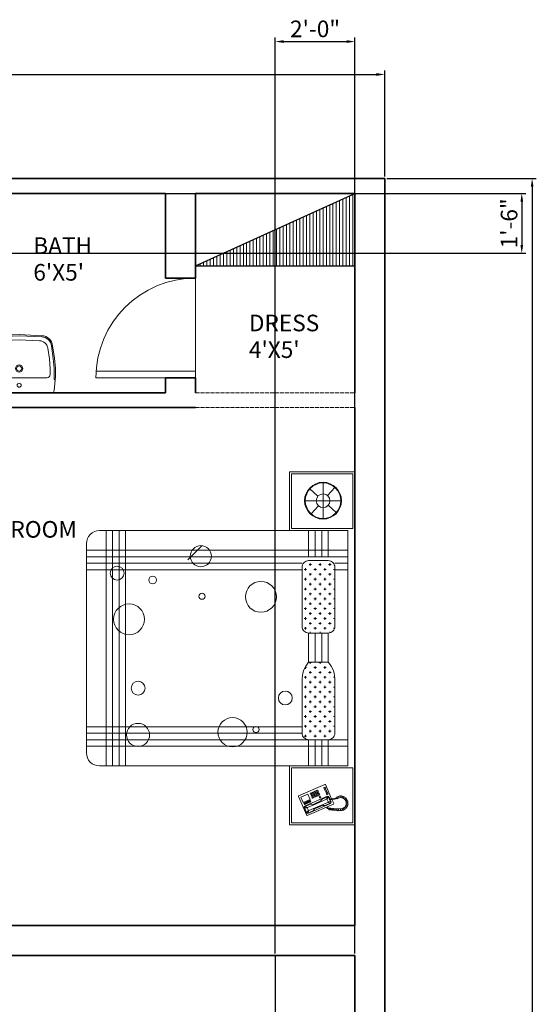
# Model space of a CAD drawing. Units: inches. Extents: x 1265 to 2734, y 1741 to 2595.
# Tile 10 of 10: x 2579 to 2734, y 2294 to 2590. Entities that reach past the tile are written whole.
import ezdxf

# ---------------------------------------------------------------- set-up
doc = ezdxf.new("R2010")
doc.units = ezdxf.units.IN
doc.header["$LTSCALE"] = 0.1
doc.linetypes.add('ACAD_ISO02W100', pattern=[15, 12, -3])
for name, color, linetype, lineweight in [('A-ANNO-DIMS', 2, 'Continuous', 18), ('A-AREA-IDEN', 7, 'Continuous', 18), ('A-DOOR', 3, 'Continuous', 18), ('A-FLOR-CASE', 33, 'Continuous', 25), ('A-FLOR-CASE-PATT', 252, 'Continuous', 13), ('A-FLOR-FIXT', 9, 'Continuous', 18), ('A-WALL', 7, 'Continuous', 35), ('A-WALL-OVHD', 7, 'ACAD_ISO02W100', 18), ('C-PROP', 7, 'Continuous', 35), ('Furniture', 8, 'Continuous', 15)]:
    doc.layers.add(name, color=color, linetype=linetype, lineweight=lineweight)
doc.styles.get("Standard").update_dxf_attribs({"font": 'arial.ttf', "height": 5})
doc.dimstyles.new('ISO-25', dxfattribs={"dimtxt": 5, "dimasz": 2.5, "dimexe": 1.25, "dimexo": 0.625, "dimtad": 1, "dimlunit": 3, "dimtxsty": 'Standard', "dimcen": 2.5, "dimadec": 0, "dimazin": 0, "dimtfac": 1, "dimtmove": 0, "dimatfit": 3, "dimfxl": 1, "dimarcsym": 0})

# ---------------------------------------------------------------- blocks, each defined once
blk = doc.blocks.new('*D2')
at = {"layer": 'A-ANNO-DIMS', "color": 0, "lineweight": -2, "transparency": 16777216}
for p, q in [((2328.6, 2543.28), (2328.6, 2575.24)), ((2331.1, 2573.99), (2686.1, 2573.99)), ((2688.6, 2543.28), (2688.6, 2575.24))]:
    blk.add_line(p, q, dxfattribs=at)
at = {"layer": 'A-ANNO-DIMS', "color": 0, "lineweight": 100, "transparency": 16777216}
for points in [[(2331.1, 2574.41), (2331.1, 2573.57), (2328.6, 2573.99)], [(2686.1, 2574.41), (2686.1, 2573.57), (2688.6, 2573.99)]]:
    blk.add_solid(points, dxfattribs=at)
at = {"layer": 'Defpoints', "color": 0, "lineweight": 100, "transparency": 16777216}
for p in [(2688.6, 2573.99), (2328.6, 2542.66), (2688.6, 2542.66)]:
    blk.add_point(p, dxfattribs=at)
at = {"layer": 'A-ANNO-DIMS', "color": 0, "transparency": 16777216, "insert": (2508.6, 2577.17), "char_height": 5, "attachment_point": 5}
blk.add_mtext("30'", dxfattribs=at)
blk = doc.blocks.new('*D3')
at = {"layer": 'A-ANNO-DIMS', "color": 0, "lineweight": -2, "transparency": 16777216}
for p, q in [((2689.23, 2542.66), (2734.23, 2542.66)), ((2732.98, 2540.16), (2732.98, 1789.16)), ((2689.23, 1786.66), (2734.23, 1786.66))]:
    blk.add_line(p, q, dxfattribs=at)
at = {"layer": 'A-ANNO-DIMS', "color": 0, "lineweight": 100, "transparency": 16777216}
for points in [[(2732.56, 2540.16), (2733.39, 2540.16), (2732.98, 2542.66)], [(2732.56, 1789.16), (2733.39, 1789.16), (2732.98, 1786.66)]]:
    blk.add_solid(points, dxfattribs=at)
at = {"layer": 'Defpoints', "color": 0, "lineweight": 100, "transparency": 16777216}
for p in [(2688.6, 2542.66), (2688.6, 1786.66), (2732.98, 1786.66)]:
    blk.add_point(p, dxfattribs=at)
at = {"layer": 'A-ANNO-DIMS', "color": 0, "transparency": 16777216, "insert": (2729.8, 2164.66), "char_height": 5, "attachment_point": 5, "rotation": 90}
blk.add_mtext("63'", dxfattribs=at)
blk = doc.blocks.new('DOOR-SWING-30IN')
for p, q in [((30, 0), (30, 30)), ((0.07, 2), (30, 2)), ((0, 0), (30, 0))]:
    blk.add_line(p, q)
blk.add_arc((30, 0), 30, 90, 180)
blk = doc.blocks.new('BASIN-WALL')
for p, q in [((10.93, 17.5), (4.12, 17.17)), ((10.93, 17.15), (4.13, 16.82)), ((10.93, 15.93), (4.76, 15.64)), ((17.75, 17.17), (10.93, 17.5)), ((17.73, 16.82), (10.93, 17.15)), ((17.1, 15.64), (10.93, 15.93)), ((0.84, 14.15), (0.29, 10.37)), ((1.19, 14.1), (0.64, 10.33)), ((2.31, 13.42), (1.84, 10.18)), ((20.02, 10.18), (19.55, 13.42)), ((21.22, 10.33), (20.67, 14.1)), ((21.57, 10.37), (21.02, 14.15)), ((0.29, 10.37), (0, 7.28)), ((0.64, 10.33), (0.35, 7.26)), ((1.84, 10.18), (1.56, 7.21)), ((20.3, 7.21), (20.02, 10.18)), ((21.52, 7.26), (21.22, 10.33)), ((21.86, 7.28), (21.57, 10.37)), ((0, 7.28), (0.02, 4.85)), ((0.35, 7.26), (0.43, 4.17)), ((1.56, 7.21), (1.57, 5.54)), ((20.29, 5.54), (20.3, 7.21)), ((21.43, 4.17), (21.52, 7.26)), ((21.85, 4.85), (21.86, 7.28)), ((0.02, 4.85), (0.4, 0.63)), ((19.25, 4.5), (2.61, 4.5)), ((21.85, 4.85), (21.46, 0.63)), ((20.77, 0), (1.09, 0))]:
    blk.add_line(p, q)
for centre, radius in [((10.93, 7.28), 1.13), ((10.93, 7.28), 0.78), ((10.93, 2.25), 0.606)]:
    blk.add_circle(centre, radius)
for centre, radius, start, end in [((4.28, 13.71), 3.46, 92.7439, 172.7579), ((4.29, 13.7), 3.12, 92.8009, 172.815), ((4.89, 13.04), 2.6, 92.7439, 171.7186), ((16.98, 13.04), 2.6, 8.2775, 87.2561), ((17.58, 13.71), 3.12, 7.2421, 87.2561), ((17.58, 13.71), 3.46, 7.2421, 87.2561), ((0.09, 4.16), 0.346, 275.1819, 0.429), ((2.61, 5.54), 1.04, 180.429, 270), ((19.25, 5.54), 1.04, 270, 359.571), ((21.78, 4.16), 0.346, 179.571, 264.8181), ((1.09, 0.69), 0.693, 185.1819, 270), ((20.77, 0.69), 0.693, 270, 354.8181)]:
    blk.add_arc(centre, radius, start, end)
blk = doc.blocks.new('BED-DOUBLE-WITH-NIGHTSTANDS')
h = blk.add_hatch()
h.set_pattern_fill('CROSS', color=256, scale=5.9055, angle=450, style=0)
h.set_pattern_definition([(90, (-724.7185, -618.2252), (1.476375, 1.476375), [0.7381875, -2.2145625]), (360, (-725.0876, -617.8561), (1.476375, -1.476375), [0.7381875, -2.2145625])])
h.paths.add_polyline_path([(13.93, 48.57), (8.02, 48.57, 0.414214), (6.06, 46.6), (6.06, 28.74, 0.414214), (8.02, 26.77), (13.93, 26.77, 0.414214), (15.9, 28.74), (15.9, 46.6, 0.414214)])
h.paths.add_polyline_path([(6.06, 62.99, 0.19223), (8.02, 57.33), (13.93, 57.33, 0.19223), (15.9, 62.99), (15.9, 78.74, 0.414214), (13.93, 80.71), (8.02, 80.71, 0.414214), (6.06, 78.74)])
for p, q in [((0, 0), (0, 106.3)), ((19.69, 106.3), (0, 106.3)), ((19.09, 105.71), (0.59, 105.71)), ((0.59, 105.71), (0.59, 89.17)), ((19.09, 105.71), (19.09, 89.17)), ((19.69, 106.3), (19.69, 88.58)), ((2.23, 100.67), (2.3, 100.88)), ((2.3, 100.88), (2.69, 100.86)), ((2.44, 101.15), (2.63, 101.34)), ((2.69, 100.86), (2.44, 101.15)), ((2.9, 100.92), (2.62, 100.19)), ((2.63, 101.34), (3.06, 101.2)), ((2.89, 101.55), (3.11, 101.7)), ((3.06, 101.2), (2.89, 101.55)), ((3.69, 101.46), (2.9, 100.92)), ((3.11, 101.7), (3.41, 101.48)), ((3.36, 101.88), (3.67, 101.95)), ((3.41, 101.48), (3.36, 101.88)), ((3.67, 101.95), (3.81, 101.64)), ((4.95, 101.56), (3.69, 101.46)), ((3.81, 101.64), (3.94, 101.98)), ((3.94, 101.98), (4.24, 102.02)), ((4.24, 102.02), (4.39, 101.64)), ((4.37, 102.03), (4.76, 102.08)), ((4.39, 101.64), (4.37, 102.03)), ((4.76, 102.08), (4.88, 101.72)), ((4.88, 101.72), (5.13, 102.07)), ((5.79, 101.48), (4.95, 101.56)), ((5.13, 102.07), (5.37, 102.03)), ((5.37, 102.03), (5.42, 101.66)), ((5.42, 101.66), (5.65, 101.97)), ((5.65, 101.97), (5.95, 101.95)), ((5.86, 101.55), (5.79, 101.48)), ((5.92, 101.48), (5.86, 101.55)), ((6.5, 101.45), (5.92, 101.48)), ((5.95, 101.95), (5.98, 101.59)), ((5.98, 101.59), (6.16, 101.92)), ((6.16, 101.92), (6.47, 101.91)), ((14.35, 103.55), (6.45, 100.09)), ((6.47, 101.91), (6.46, 101.54)), ((6.46, 101.54), (6.62, 101.9)), ((7.29, 101.35), (6.5, 101.45)), ((6.62, 101.9), (6.85, 101.89)), ((6.85, 101.89), (6.89, 101.51)), ((6.89, 101.51), (7.15, 101.84)), ((7.15, 101.84), (7.36, 101.82)), ((7.73, 101.29), (7.29, 101.35)), ((14.21, 102.94), (7.34, 99.94)), ((7.36, 101.82), (7.4, 101.48)), ((7.4, 101.48), (7.62, 101.8)), ((7.62, 101.8), (7.77, 101.81)), ((7.79, 101.48), (7.73, 101.29)), ((7.77, 101.81), (7.86, 101.7)), ((7.84, 101.37), (7.79, 101.48)), ((7.94, 101.33), (7.84, 101.37)), ((7.86, 101.7), (7.96, 101.49)), ((8.11, 101.22), (7.94, 101.33)), ((7.96, 101.49), (8.25, 101.43)), ((8.26, 101.14), (8.11, 101.22)), ((11.28, 100.91), (8.18, 99.56)), ((8.25, 101.43), (8.4, 101.32)), ((8.4, 100.95), (8.26, 101.14)), ((8.4, 101.32), (8.57, 101.02)), ((10.11, 100.6), (11.2, 101.08)), ((11.78, 101.33), (11.2, 101.08)), ((11.28, 100.91), (13.85, 102.03)), ((11.68, 99.99), (14.26, 101.12)), ((12.15, 101.56), (11.78, 101.33)), ((12.36, 101.86), (12.15, 101.56)), ((12.6, 102.1), (12.36, 101.86)), ((14.14, 102.78), (12.6, 102.1)), ((15, 100.83), (13.45, 100.15)), ((14.14, 102.78), (13.85, 102.03)), ((13.85, 102.03), (13.99, 102.03)), ((13.99, 102.03), (14.61, 102.64)), ((13.99, 102.03), (14.34, 101.23)), ((14.4, 102.82), (14.14, 102.78)), ((14.62, 102.78), (14.21, 102.94)), ((14.26, 101.12), (14.34, 101.23)), ((15, 100.83), (14.26, 101.12)), ((14.34, 101.23), (15.21, 101.26)), ((14.52, 103.48), (14.35, 103.55)), ((14.61, 102.64), (14.4, 102.82)), ((17.02, 97.76), (14.52, 103.48)), ((15.21, 101.26), (14.61, 102.64)), ((15.37, 101.06), (14.62, 102.78)), ((15.2, 100.99), (15, 100.83)), ((15.19, 100.71), (15.37, 101.06)), ((15.21, 101.26), (15.2, 100.99)), ((2.06, 100.15), (2.14, 100.41)), ((2.46, 100.04), (2.06, 100.15)), ((2.09, 99.7), (2.1, 99.92)), ((2.44, 99.53), (2.09, 99.7)), ((2.1, 99.92), (2.46, 100.04)), ((2.13, 99.38), (2.44, 99.53)), ((2.17, 99.14), (2.13, 99.38)), ((2.14, 100.41), (2.51, 100.41)), ((2.59, 99.17), (2.17, 99.14)), ((2.51, 100.41), (2.23, 100.67)), ((2.29, 98.95), (2.59, 99.17)), ((2.4, 98.76), (2.29, 98.95)), ((2.78, 98.76), (2.4, 98.76)), ((2.53, 98.47), (2.78, 98.76)), ((2.71, 98.26), (2.53, 98.47)), ((2.62, 100.19), (2.62, 99.39)), ((2.62, 99.39), (2.99, 98.72)), ((3.07, 98.46), (2.71, 98.26)), ((2.96, 98.08), (3.07, 98.46)), ((3.2, 97.92), (2.96, 98.08)), ((2.99, 98.72), (3.58, 98.25)), ((3.49, 98.1), (3.2, 97.92)), ((3.41, 97.75), (3.49, 98.1)), ((3.58, 98.25), (4.33, 98.05)), ((3.95, 97.97), (3.7, 97.67)), ((4.03, 97.59), (3.95, 97.97)), ((4.33, 98.05), (5.08, 98.31)), ((4.48, 97.99), (4.36, 97.56)), ((4.67, 97.64), (4.48, 97.99)), ((5.05, 98.16), (5, 97.75)), ((5.26, 97.85), (5.05, 98.16)), ((5.08, 98.31), (5.33, 98.48)), ((5.53, 98), (5.26, 97.85)), ((5.33, 98.48), (5.57, 98.34)), ((5.6, 98.18), (5.53, 98)), ((5.57, 98.34), (5.87, 98.48)), ((5.68, 98.18), (5.6, 98.18)), ((5.98, 98.32), (5.68, 98.18)), ((5.87, 98.48), (6.16, 98.57)), ((6.58, 98.42), (5.98, 98.32)), ((6.16, 98.57), (6.77, 98.66)), ((6.45, 100.09), (6.38, 99.93)), ((6.38, 99.93), (6.92, 98.7)), ((7.23, 98.53), (6.58, 98.42)), ((6.77, 98.66), (7.17, 98.75)), ((7.01, 98.5), (8.89, 94.2)), ((7.34, 99.94), (7.12, 99.5)), ((7.12, 99.5), (7.41, 98.83)), ((7.17, 98.75), (7.65, 98.91)), ((7.23, 99.41), (7.24, 99.69)), ((8.1, 99.45), (7.23, 99.41)), ((7.47, 98.85), (7.23, 99.41)), ((7.72, 98.74), (7.23, 98.53)), ((7.24, 99.69), (7.44, 99.85)), ((7.44, 99.85), (8.99, 100.52)), ((7.44, 99.85), (8.18, 99.56)), ((7.49, 98.64), (7.84, 97.84)), ((7.83, 98.04), (7.55, 98.67)), ((7.65, 98.91), (7.72, 98.74)), ((8.45, 98.65), (7.83, 98.04)), ((7.83, 98.04), (8.04, 97.86)), ((8.04, 97.86), (8.3, 97.9)), ((8.18, 99.56), (8.1, 99.45)), ((8.1, 99.45), (8.45, 98.65)), ((8.26, 97.68), (15.19, 100.71)), ((8.3, 97.9), (8.59, 98.64)), ((8.3, 97.9), (9.84, 98.58)), ((8.59, 98.64), (8.45, 98.65)), ((11.68, 99.99), (8.59, 98.64)), ((8.99, 100.52), (9.33, 100.53)), ((9.33, 100.53), (9.69, 100.49)), ((9.69, 100.49), (10.11, 100.6)), ((9.84, 98.58), (10.08, 98.82)), ((10.08, 98.82), (10.29, 99.11)), ((10.58, 98.29), (10.24, 98.14)), ((10.24, 98.14), (10.44, 97.68)), ((10.29, 99.11), (10.66, 99.34)), ((10.78, 97.83), (10.58, 98.29)), ((10.66, 99.34), (11.75, 99.82)), ((12.33, 100.07), (11.75, 99.82)), ((12.19, 98.03), (11.85, 97.88)), ((11.85, 97.88), (12, 97.54)), ((12.34, 97.69), (12.19, 98.03)), ((12.75, 100.19), (12.33, 100.07)), ((12.82, 98.31), (12.48, 98.16)), ((12.48, 98.16), (12.63, 97.82)), ((12.63, 97.82), (12.97, 97.97)), ((13.11, 100.14), (12.75, 100.19)), ((12.97, 97.97), (12.82, 98.31)), ((13.45, 100.15), (13.11, 100.14)), ((13.3, 99.4), (13.47, 99.48)), ((13.5, 98.95), (13.3, 99.4)), ((15.58, 99.65), (13.46, 98.72)), ((13.46, 98.72), (14.19, 97.06)), ((13.47, 99.48), (13.67, 99.02)), ((13.67, 99.02), (13.5, 98.95)), ((13.64, 99.55), (13.81, 99.63)), ((13.84, 99.1), (13.64, 99.55)), ((13.81, 99.63), (14.01, 99.17)), ((14.01, 99.17), (13.84, 99.1)), ((13.99, 99.7), (14.16, 99.78)), ((14.19, 99.25), (13.99, 99.7)), ((14.16, 99.78), (14.36, 99.32)), ((14.36, 99.32), (14.19, 99.25)), ((14.19, 97.06), (16.3, 97.99)), ((14.33, 99.85), (14.5, 99.93)), ((14.53, 99.4), (14.33, 99.85)), ((14.5, 99.93), (14.7, 99.47)), ((14.7, 99.47), (14.53, 99.4)), ((14.67, 100), (14.85, 100.08)), ((14.87, 99.55), (14.67, 100)), ((14.85, 100.08), (15.05, 99.62)), ((15.05, 99.62), (14.87, 99.55)), ((15.02, 100.16), (15.19, 100.23)), ((15.22, 99.7), (15.02, 100.16)), ((15.19, 100.23), (15.39, 99.77)), ((15.39, 99.77), (15.22, 99.7)), ((16.3, 97.99), (15.58, 99.65)), ((3.7, 97.67), (3.41, 97.75)), ((4.36, 97.56), (4.03, 97.59)), ((5, 97.75), (4.67, 97.64)), ((7.84, 97.84), (8.26, 97.68)), ((8.09, 97.13), (8.43, 97.28)), ((8.34, 96.55), (8.09, 97.13)), ((8.68, 96.7), (8.34, 96.55)), ((8.43, 97.28), (8.68, 96.7)), ((8.44, 96.33), (8.78, 96.48)), ((8.69, 95.75), (8.44, 96.33)), ((9.03, 95.9), (8.69, 95.75)), ((8.78, 96.48), (9.03, 95.9)), ((8.79, 95.52), (9.13, 95.67)), ((9.04, 94.95), (8.79, 95.52)), ((9.38, 95.1), (9.04, 94.95)), ((9.05, 94.14), (16.96, 97.59)), ((9.13, 95.67), (9.38, 95.1)), ((10.44, 97.68), (10.78, 97.83)), ((10.93, 97.48), (10.59, 97.33)), ((10.59, 97.33), (10.74, 96.99)), ((10.74, 96.99), (11.08, 97.14)), ((11.18, 96.91), (10.84, 96.76)), ((10.84, 96.76), (10.99, 96.42)), ((11.08, 97.14), (10.93, 97.48)), ((10.99, 96.42), (11.33, 96.57)), ((11.43, 96.34), (11.09, 96.19)), ((11.09, 96.19), (11.24, 95.84)), ((11.33, 96.57), (11.18, 96.91)), ((11.56, 97.76), (11.22, 97.61)), ((11.22, 97.61), (11.37, 97.26)), ((11.24, 95.84), (11.58, 95.99)), ((11.37, 97.26), (11.71, 97.42)), ((11.58, 95.99), (11.43, 96.34)), ((11.81, 97.19), (11.47, 97.04)), ((11.47, 97.04), (11.62, 96.69)), ((11.71, 97.42), (11.56, 97.76)), ((11.62, 96.69), (11.96, 96.84)), ((12.06, 96.61), (11.72, 96.46)), ((11.72, 96.46), (11.87, 96.12)), ((11.96, 96.84), (11.81, 97.19)), ((11.87, 96.12), (12.21, 96.27)), ((12, 97.54), (12.34, 97.69)), ((12.21, 96.27), (12.06, 96.61)), ((12.44, 97.46), (12.1, 97.31)), ((12.1, 97.31), (12.25, 96.97)), ((12.25, 96.97), (12.59, 97.12)), ((12.69, 96.89), (12.35, 96.74)), ((12.35, 96.74), (12.5, 96.39)), ((12.59, 97.12), (12.44, 97.46)), ((12.5, 96.39), (12.84, 96.55)), ((12.84, 96.55), (12.69, 96.89)), ((13.07, 97.74), (12.73, 97.59)), ((12.73, 97.59), (12.88, 97.24)), ((12.88, 97.24), (13.22, 97.39)), ((13.32, 97.16), (12.98, 97.01)), ((12.98, 97.01), (13.13, 96.67)), ((13.22, 97.39), (13.07, 97.74)), ((13.13, 96.67), (13.47, 96.82)), ((13.47, 96.82), (13.32, 97.16)), ((16.96, 97.59), (17.02, 97.76)), ((8.89, 94.2), (9.05, 94.14)), ((19.09, 89.17), (0.59, 89.17)), ((0.59, 89.17), (19.09, 89.17)), ((2.12, 17.72), (2.12, 88.58)), ((2.12, 88.58), (76.92, 88.58)), ((80.86, 84.65), (80.86, 21.65)), ((55.34, 82.68), (55.28, 82.62)), ((6.07, 78.97), (6.07, 62.76)), ((6.07, 44.57), (6.06, 44.56)), ((6.07, 46.84), (6.07, 28.51)), ((50.36, 26.51), (46.1, 22.26)), ((19.09, 17.13), (0.59, 17.13)), ((0.59, 0.59), (0.59, 17.13)), ((76.92, 17.72), (2.12, 17.72)), ((19.09, 0.59), (19.09, 17.13)), ((19.69, 0), (19.69, 17.72)), ((8.07, 10.1), (5.65, 12.3)), ((9.61, 8.71), (9.61, 14.05)), ((11, 10.24), (13.2, 12.67)), ((9.61, 8.71), (4.26, 8.71)), ((8.22, 7.18), (6.02, 4.75)), ((9.61, 8.71), (14.95, 8.71)), ((9.61, 8.71), (9.61, 3.36)), ((11.14, 7.32), (13.57, 5.12)), ((19.69, 0), (0, 0)), ((19.09, 0.59), (0.59, 0.59))]:
    blk.add_line(p, q)
for points in [[(8.02, 88.58), (8.02, 80.71)], [(9.99, 80.71), (9.99, 88.58), (8.02, 88.58)], [(13.93, 80.71), (13.93, 88.58), (11.96, 88.58)], [(11.96, 88.58), (11.96, 80.71)], [(2.12, 80.71), (80.86, 80.71), (80.86, 82.68), (2.12, 82.68)], [(15.9, 76.77), (80.86, 76.77), (80.86, 78.74), (15.9, 78.74)], [(8.02, 57.33), (8.02, 48.57)], [(9.99, 48.57), (9.99, 57.33)], [(11.96, 57.33), (11.96, 48.57)], [(13.93, 48.57), (13.93, 57.33)], [(2.12, 29.53), (6.06, 29.53)], [(6.06, 27.56), (2.12, 27.56)], [(15.9, 29.53), (80.86, 29.53), (80.86, 27.56), (15.9, 27.56)], [(2.12, 25.59), (80.86, 25.59), (80.86, 23.62), (2.12, 23.62)], [(8.02, 25.59), (8.02, 17.72), (9.99, 17.72), (9.99, 25.59)], [(11.96, 25.59), (11.96, 17.72), (13.93, 17.72), (13.93, 25.59)]]:
    blk.add_lwpolyline(points)
for points in [[(69.05, 88.58), (69.05, 17.72), (71.02, 17.72), (71.02, 88.58)], [(72.98, 88.58), (72.98, 17.72), (74.95, 17.72), (74.95, 88.58)]]:
    blk.add_lwpolyline(points, close=True)
for points in [[(15.9, 62.99), (15.9, 78.74, 0.414214), (13.93, 80.71), (8.02, 80.71, 0.414214), (6.06, 78.74), (6.06, 62.99, 0.19223), (8.02, 57.33), (13.93, 57.33, 0.19223)], [(15.9, 28.74), (15.9, 46.6, 0.414214), (13.93, 48.57), (8.02, 48.57, 0.414214), (6.06, 46.6), (6.06, 28.74, 0.414214), (8.02, 26.77), (13.93, 26.77, 0.414214)]]:
    blk.add_lwpolyline(points, format="xyb", close=True)
for centre, radius in [((36.86, 78.44), 4.41), ((65.32, 79.25), 3.48), ((29.81, 77.62), 0.925), ((20.97, 68.13), 2.09), ((65.3, 65.16), 2.09), ((68.02, 44.43), 4.65), ((28.31, 37.66), 4.65), ((46.05, 37.48), 0.925), ((60.91, 32.6), 1.14), ((71.58, 30.51), 2.09), ((46.4, 25.43), 3.19), ((9.61, 8.71), 5.54), ((9.61, 8.71), 5.34), ((9.61, 8.71), 2.07)]:
    blk.add_circle(centre, radius)
for centre, start, end in [((76.92, 84.65), 0, 90), ((76.92, 21.65), 270, 0)]:
    blk.add_arc(centre, 3.94, start, end)
blk = doc.blocks.new('*D44')
at = {"layer": 'A-ANNO-DIMS', "color": 0, "lineweight": -2, "transparency": 16777216}
for p, q in [((2446.23, 2538.16), (2731.1, 2538.16)), ((2729.85, 2535.66), (2729.85, 2522.66)), ((2446.23, 2520.16), (2731.1, 2520.16))]:
    blk.add_line(p, q, dxfattribs=at)
at = {"layer": 'A-ANNO-DIMS', "color": 0, "lineweight": 100, "transparency": 16777216}
for points in [[(2729.44, 2535.66), (2730.27, 2535.66), (2729.85, 2538.16)], [(2729.44, 2522.66), (2730.27, 2522.66), (2729.85, 2520.16)]]:
    blk.add_solid(points, dxfattribs=at)
at = {"layer": 'Defpoints', "color": 0, "lineweight": 100, "transparency": 16777216}
for p in [(2445.6, 2538.16), (2445.6, 2520.16), (2729.85, 2520.16)]:
    blk.add_point(p, dxfattribs=at)
at = {"layer": 'A-ANNO-DIMS', "color": 0, "transparency": 16777216, "insert": (2726.67, 2529.16), "char_height": 5, "attachment_point": 5, "rotation": 90}
blk.add_mtext('1\'-6"', dxfattribs=at)
blk = doc.blocks.new('*D46')
at = {"layer": 'A-ANNO-DIMS', "color": 0, "lineweight": -2, "transparency": 16777216}
for p, q in [((2655.6, 2309.28), (2655.6, 2585.16)), ((2658.1, 2583.91), (2677.1, 2583.91)), ((2679.6, 2309.28), (2679.6, 2585.16))]:
    blk.add_line(p, q, dxfattribs=at)
at = {"layer": 'A-ANNO-DIMS', "color": 0, "lineweight": 100, "transparency": 16777216}
for points in [[(2658.1, 2584.32), (2658.1, 2583.49), (2655.6, 2583.91)], [(2677.1, 2584.32), (2677.1, 2583.49), (2679.6, 2583.91)]]:
    blk.add_solid(points, dxfattribs=at)
at = {"layer": 'Defpoints', "color": 0, "lineweight": 100, "transparency": 16777216}
for p in [(2679.6, 2583.91), (2655.6, 2308.66), (2679.6, 2308.66)]:
    blk.add_point(p, dxfattribs=at)
at = {"layer": 'A-ANNO-DIMS', "color": 0, "transparency": 16777216, "insert": (2667.6, 2587.08), "char_height": 5, "attachment_point": 5}
blk.add_mtext('2\'-0"', dxfattribs=at)

msp = doc.modelspace()

# ---------------------------------------------------------------- hatches: boundary and pattern name
at = {"layer": 'A-FLOR-CASE-PATT'}
h = msp.add_hatch(dxfattribs=at)
h.set_pattern_fill('ANSI31', color=256, scale=0.3149606, angle=45, style=0)
h.paths.add_polyline_path([(2631.602, 2516.413), (2679.602, 2516.413), (2679.602, 2538.157)])

# ---------------------------------------------------------------- linework, layer by layer
at = {"layer": 'A-FLOR-CASE'}
for p, q in [((2631.602, 2516.413), (2679.602, 2538.157)), ((2631.602, 2535.892), (2631.602, 2516.413)), ((2631.602, 2516.413), (2679.602, 2516.413)), ((2655.602, 2308.657), (2655.602, 2248.657))]:
    msp.add_line(p, q, dxfattribs=at)
at = {"layer": 'A-WALL'}
for p, q in [((2550.602, 2538.157), (2622.602, 2538.157)), ((2622.602, 2512.657), (2622.602, 2538.157)), ((2631.602, 2538.157), (2679.602, 2538.157)), ((2631.602, 2512.657), (2631.602, 2538.157)), ((2679.602, 2538.157), (2679.602, 2478.157)), ((2631.602, 2512.657), (2622.602, 2512.657)), ((2622.602, 2478.157), (2622.602, 2482.657)), ((2631.602, 2482.657), (2622.602, 2482.657)), ((2631.602, 2478.157), (2631.602, 2482.657)), ((2550.602, 2478.157), (2622.602, 2478.157)), ((2490.602, 2473.657), (2631.602, 2473.657)), ((2679.602, 2473.657), (2679.602, 2317.657)), ((2531.102, 2317.657), (2679.602, 2317.657)), ((2547.602, 2308.657), (2679.602, 2308.657)), ((2679.602, 2308.657), (2679.602, 2224.657))]:
    msp.add_line(p, q, dxfattribs=at)
at = {"layer": 'A-WALL-OVHD'}
for p, q in [((2631.602, 2478.157), (2679.602, 2478.157)), ((2631.602, 2473.657), (2679.602, 2473.657))]:
    msp.add_line(p, q, dxfattribs=at)
at = {"layer": 'C-PROP'}
for p, q in [((2328.602, 2542.657), (2688.602, 2542.657)), ((2688.602, 2542.657), (2688.602, 1786.657))]:
    msp.add_line(p, q, dxfattribs=at)

# ---------------------------------------------------------------- block references
at = {"layer": 'A-DOOR'}
msp.add_blockref('DOOR-SWING-30IN', (2601.602, 2482.657), dxfattribs=at)
at = {"layer": 'A-FLOR-FIXT'}
msp.add_blockref('BASIN-WALL', (2567.559, 2478.157), dxfattribs=at)
at = {"layer": 'Furniture', "rotation": 180}
msp.add_blockref('BED-DOUBLE-WITH-NIGHTSTANDS', (2679.603, 2454.351), dxfattribs=at)

# ---------------------------------------------------------------- texts
at = {"layer": 'A-AREA-IDEN'}
for s, p in [('BATH', (2582.754, 2519.942)), ("6'X5'", (2582.754, 2511.91)), ('DRESS', (2647.674, 2496.653)), ("4'X5'", (2647.674, 2488.621)), ('MASTER BED ROOM', (2533.419, 2434.508))]:
    msp.add_text(s, height=5, dxfattribs=at).set_placement(p)

# ---------------------------------------------------------------- dimensions: what is measured, and where the dimension line sits
at = {"layer": 'A-ANNO-DIMS'}
for base, p1, p2, override, picture, middle in [((2679.602, 2583.907), (2655.602, 2308.657), (2679.602, 2308.657), {"dimdec": 1, "dimlfac": 1, "dimrnd": 0, "dimzin": 1, "dimdsep": 46, "dimlunit": 4, "dimfrac": 2}, '*D46', (2667.602, 2587.085)), ((2688.602, 2573.99), (2328.602, 2542.657), (2688.602, 2542.657), {"dimclrd": 0, "dimclre": 0, "dimclrt": 0}, '*D2', (2508.602, 2577.169))]:
    dim = msp.add_linear_dim(base=base, p1=p1, p2=p2, dimstyle='ISO-25', override=override, dxfattribs=at)
    dim.commit()
    dim.dimension.update_dxf_attribs({"geometry": picture, "text_midpoint": middle})
for base, p1, p2, override, picture, middle in [((2732.978, 1786.657), (2688.602, 2542.657), (2688.602, 1786.657), {"dimclrd": 0, "dimclre": 0, "dimclrt": 0}, '*D3', (2729.798, 2164.657)), ((2729.852, 2520.157), (2445.602, 2538.157), (2445.602, 2520.157), {"dimdec": 1, "dimlfac": 1, "dimrnd": 0, "dimzin": 1, "dimdsep": 46, "dimlunit": 4, "dimfrac": 2}, '*D44', (2726.675, 2529.157))]:
    dim = msp.add_linear_dim(base=base, p1=p1, p2=p2, angle=90, dimstyle='ISO-25', override=override, dxfattribs=at)
    dim.commit()
    dim.dimension.update_dxf_attribs({"geometry": picture, "text_midpoint": middle})

doc.saveas('drawing.dxf')
